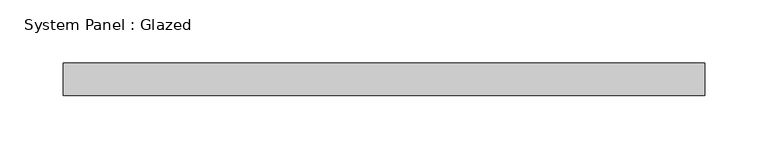
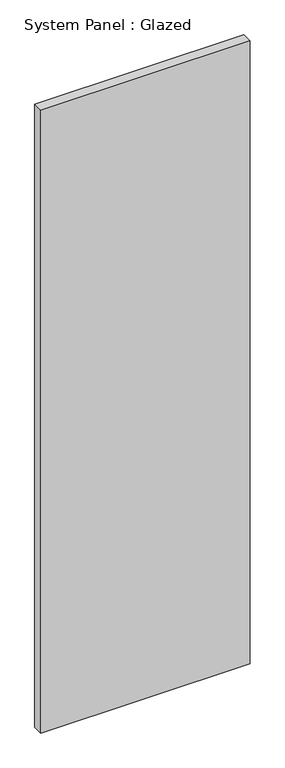
"""IFC4 building model written with IfcOpenShell, lengths in millimetres: plate geometry, System Panel : Glazed."""

from ifc_helpers import new_model, si_unit, origin, origin_with_axes, place, context, project, spatial, polyline, outline, extrude, source, transform, mapped, element, save


def system_panel_glazed_4d5622a9(model_context):
    return source(origin(), model_context, "Body", "SweptSolid", [
        extrude(outline(polyline([(252.9416667, 19.05), (-252.9416667, 19.05), (-252.9416667, 44.45), (252.9416667, 44.45), (252.9416667, 19.05)])), origin_with_axes(), (0.0, 0.0, 1.0), 1591.7125392),
    ])


if __name__ == "__main__":
    model = new_model("IFC4")
    model_context = context("Model", 3, world=origin())
    ifc_project = project(units=[si_unit("LENGTHUNIT", "METRE", prefix="MILLI")], contexts=[model_context])
    site = spatial("IfcSite", under=ifc_project)
    building = spatial("IfcBuilding", under=site)
    placement = place(None, origin())
    system_panel_glazed_shape = system_panel_glazed_4d5622a9(model_context)
    element("IfcPlate", 1, ObjectType="System Panel : Glazed", at=placement, inside=building, context=model_context, shape_type="MappedRepresentation", body=[
        mapped(system_panel_glazed_shape, transform((0.0, 0.0, 0.0), x_axis=(1.0, 0.0, 0.0), y_axis=(0.0, 1.0, 0.0), z_axis=(0.0, 0.0, 1.0))),
    ])
    save(model, "model.ifc")

# Revit data of these elements
# Type "System Panel : Glazed"
#   Construction Type Id = "GSP4R"
#   Analytic Construction = "1/8 in Pilkington single glazing"
#   Visual Light Transmittance = 0.9
#   Solar Heat Gain Coefficient = 0.86
#   Heat Transfer Coefficient (U) = 1.18115 BTU/(h·ft²·°F)
#   Define Thermal Properties by = 1
# Element 1 (IfcPlate, "System Panel : Glazed")
#   Materials on its faces: "Glass"
# Materials
#   "Glass": class "Glass", colour RGB 0 128 192, transparency 0.75, Description = "Soda Lime Glass", Cost = 0
